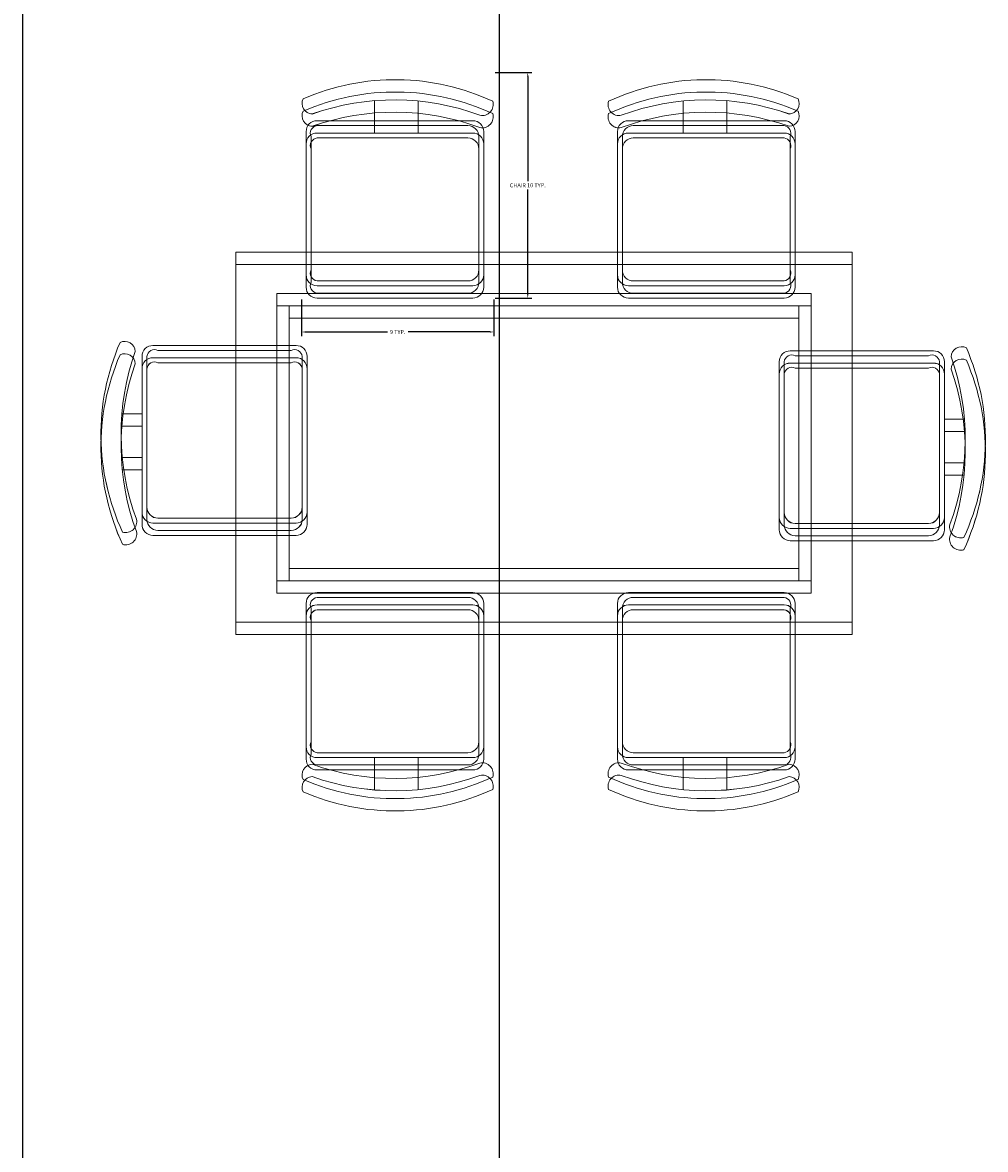
# Model space of a CAD drawing. Units: inches. Extents: x 2063 to 2617, y 1299 to 2210.
# Tile 18 of 22: x 2388 to 2431, y 1889 to 1939. Entities that reach past the tile are written whole.
import ezdxf

# ---------------------------------------------------------------- set-up
doc = ezdxf.new("R2010")
doc.units = ezdxf.units.IN
doc.layers.add('A-ANNO-DIMS', color=2, linetype='Continuous', lineweight=18)
doc.layers.add('A-FURN', color=8, linetype='Continuous', lineweight=18)
doc.styles.get("Standard").update_dxf_attribs({"font": 'arial.ttf'})
doc.dimstyles.get("Standard").update_dxf_attribs({"dimtxt": 0.18, "dimasz": 0.18, "dimexe": 0.18, "dimexo": 0.0625, "dimgap": 0.09, "dimtad": 0, "dimtih": 1, "dimtoh": 1, "dimdec": 4, "dimzin": 0, "dimdsep": 46, "dimtxsty": 'Standard', "dimcen": 0.09, "dimadec": 0, "dimazin": 0, "dimtfac": 1, "dimtdec": 4, "dimtofl": 0, "dimtmove": 0, "dimatfit": 3, "dimfxl": 1, "dimtolj": 1, "dimtzin": 0, "dimarcsym": 0})

# ---------------------------------------------------------------- blocks, each defined once
blk = doc.blocks.new('TABLE-DINING')
for points in [[(0, 17.017), (27.446, 17.017), (27.446, 0.549), (0, 0.549)], [(0, 17.017), (27.446, 17.017), (27.446, 0.549), (0, 0.549)], [(0, 17.016), (27.446, 17.016), (27.446, 0.549), (0, 0.549)], [(0, 17.016), (27.446, 17.016), (27.446, 0.549), (0, 0.549)], [(0, 16.468), (27.446, 16.468), (27.446, 0), (0, 0)], [(0, 16.468), (27.446, 16.468), (27.446, 0), (0, 0)], [(0, 16.467), (27.446, 16.467), (27.446, 0), (0, 0)], [(0, 16.467), (27.446, 16.467), (27.446, 0), (0, 0)], [(1.83, 15.187), (25.616, 15.187), (25.616, 2.379), (1.83, 2.379)], [(1.83, 15.187), (25.616, 15.187), (25.616, 2.379), (1.83, 2.379)], [(1.83, 15.187), (25.616, 15.187), (25.616, 2.379), (1.83, 2.379)], [(1.83, 15.187), (25.616, 15.187), (25.616, 2.379), (1.83, 2.379)], [(1.83, 14.638), (25.616, 14.638), (25.616, 1.83), (1.83, 1.83)], [(1.83, 14.638), (25.616, 14.638), (25.616, 1.83), (1.83, 1.83)], [(1.83, 14.638), (25.616, 14.638), (25.616, 1.83), (1.83, 1.83)], [(1.83, 14.638), (25.616, 14.638), (25.616, 1.83), (1.83, 1.83)], [(2.379, 14.638), (25.067, 14.638), (25.067, 2.928), (2.379, 2.928)], [(2.379, 14.638), (25.067, 14.638), (25.067, 2.927), (2.379, 2.927)], [(2.379, 14.638), (25.067, 14.638), (25.067, 2.928), (2.379, 2.928)], [(2.379, 14.638), (25.067, 14.638), (25.067, 2.927), (2.379, 2.927)], [(2.379, 14.089), (25.067, 14.089), (25.067, 2.379), (2.379, 2.379)], [(2.379, 14.089), (25.067, 14.089), (25.067, 2.379), (2.379, 2.379)], [(2.379, 14.089), (25.067, 14.089), (25.067, 2.379), (2.379, 2.379)], [(2.379, 14.089), (25.067, 14.089), (25.067, 2.379), (2.379, 2.379)]]:
    blk.add_lwpolyline(points, close=True)
blk = doc.blocks.new('CHAIR-DINING')
for points in [[(0.449, 8.202, -0.175809), (7.924, 8.145, 0.578392), (8.491, 8.768, 0.214524), (0.052, 8.881, 0.552014), (0.449, 8.202, -0.065079)], [(0.449, 8.201, -0.175809), (7.924, 8.145, 0.578392), (8.491, 8.767, 0.214524), (0.053, 8.881, 0.552014), (0.449, 8.201, -0.065079)], [(0.449, 8.202, -0.175809), (7.924, 8.145, 0.578392), (8.491, 8.768, 0.214524), (0.052, 8.881, 0.552014), (0.449, 8.202, -0.065079)], [(0.449, 8.201, -0.175809), (7.924, 8.145, 0.578392), (8.491, 8.767, 0.214524), (0.053, 8.881, 0.552014), (0.449, 8.201, -0.065079)], [(0.449, 7.653, -0.175809), (7.924, 7.596, 0.578392), (8.491, 8.219, 0.214524), (0.052, 8.332, 0.552014), (0.449, 7.653, -0.065079)], [(0.449, 7.652, -0.175809), (7.924, 7.596, 0.578392), (8.491, 8.218, 0.214524), (0.053, 8.332, 0.552014), (0.449, 7.652, -0.065079)], [(0.449, 7.653, -0.175809), (7.924, 7.596, 0.578392), (8.491, 8.219, 0.214524), (0.052, 8.332, 0.552014), (0.449, 7.653, -0.065079)], [(0.449, 7.652, -0.175809), (7.924, 7.596, 0.578392), (8.491, 8.218, 0.214524), (0.053, 8.332, 0.552014), (0.449, 7.652, -0.065079)], [(5.17, 7.902), (5.17, 8.779, -0.064759)], [(5.17, 7.901), (5.17, 8.779, -0.064759)], [(5.17, 7.902), (5.17, 8.779, -0.064759)], [(5.17, 7.901), (5.17, 8.779, -0.064759)], [(5.17, 7.353), (5.17, 8.23, -0.064759)], [(5.17, 7.352), (5.17, 8.23, -0.064759)], [(5.17, 7.353), (5.17, 8.23, -0.064759)], [(5.17, 7.352), (5.17, 8.23, -0.064759)], [(7.607, 7.902), (0.667, 7.902, 0.414214), (0.182, 7.416), (0.182, 1.035, 0.414214), (0.667, 0.549), (7.607, 0.549, 0.414214), (8.093, 1.035), (8.093, 7.416, 0.414214), (7.607, 7.902)], [(7.607, 7.902), (0.667, 7.902, 0.414214), (0.182, 7.416), (0.182, 1.035, 0.414214), (0.667, 0.549), (7.607, 0.549, 0.414214), (8.093, 1.035), (8.093, 7.416, 0.414214), (7.607, 7.902)], [(7.607, 7.901), (0.667, 7.901, 0.414214), (0.182, 7.416), (0.182, 1.035, 0.414214), (0.667, 0.549), (7.607, 0.549, 0.414214), (8.093, 1.035), (8.093, 7.416, 0.414214), (7.607, 7.901)], [(7.607, 7.901), (0.667, 7.901, 0.414214), (0.182, 7.416), (0.182, 1.035, 0.414214), (0.667, 0.549), (7.607, 0.549, 0.414214), (8.093, 1.035), (8.093, 7.416, 0.414214), (7.607, 7.901)], [(7.607, 7.353), (0.667, 7.353, 0.414214), (0.182, 6.867), (0.182, 0.486, 0.414214), (0.667, 0), (7.607, 0, 0.414214), (8.093, 0.486), (8.093, 6.867, 0.414214), (7.607, 7.353)], [(7.607, 7.353), (0.667, 7.353, 0.414214), (0.182, 6.867), (0.182, 0.486, 0.414214), (0.667, 0), (7.607, 0, 0.414214), (8.093, 0.486), (8.093, 6.867, 0.414214), (7.607, 7.353)], [(7.607, 7.352), (0.667, 7.352, 0.414214), (0.182, 6.867), (0.182, 0.486, 0.414214), (0.667, 0), (7.607, 0, 0.414214), (8.093, 0.486), (8.093, 6.867, 0.414214), (7.607, 7.352)], [(7.607, 7.352), (0.667, 7.352, 0.414214), (0.182, 6.867), (0.182, 0.486, 0.414214), (0.667, 0), (7.607, 0, 0.414214), (8.093, 0.486), (8.093, 6.867, 0.414214), (7.607, 7.352)]]:
    blk.add_lwpolyline(points, format="xyb")
for points in [[(3.227, 8.795), (3.227, 7.902)], [(3.227, 8.795), (3.227, 7.901)], [(3.227, 8.795), (3.227, 7.902)], [(3.227, 8.795), (3.227, 7.901)], [(3.227, 8.246), (3.227, 7.353)], [(3.227, 8.246), (3.227, 7.352)], [(3.227, 8.246), (3.227, 7.353)], [(3.227, 8.246), (3.227, 7.352)]]:
    blk.add_lwpolyline(points)
for points in [[(0.67, 7.683), (7.388, 7.683, -0.414214), (7.874, 7.197), (7.874, 1.254, -0.414214), (7.388, 0.768), (0.67, 0.768, -0.512069), (0.4, 1.254), (0.4, 7.197, -0.512069)], [(0.67, 7.683), (7.388, 7.683, -0.414214), (7.874, 7.197), (7.874, 1.253, -0.414214), (7.388, 0.768), (0.67, 0.768, -0.512069), (0.4, 1.253), (0.4, 7.197, -0.512069)], [(0.67, 7.683), (7.388, 7.683, -0.414214), (7.874, 7.197), (7.874, 1.254, -0.414214), (7.388, 0.768), (0.67, 0.768, -0.512069), (0.4, 1.254), (0.4, 7.197, -0.512069)], [(0.67, 7.683), (7.388, 7.683, -0.414214), (7.874, 7.197), (7.874, 1.253, -0.414214), (7.388, 0.768), (0.67, 0.768, -0.512069), (0.4, 1.253), (0.4, 7.197, -0.512069)], [(0.67, 7.134), (7.388, 7.134, -0.414214), (7.874, 6.648), (7.874, 0.705, -0.414214), (7.388, 0.219), (0.67, 0.219, -0.512069), (0.4, 0.705), (0.4, 6.648, -0.512069)], [(0.67, 7.134), (7.388, 7.134, -0.414214), (7.874, 6.648), (7.874, 0.704, -0.414214), (7.388, 0.219), (0.67, 0.219, -0.512069), (0.4, 0.704), (0.4, 6.648, -0.512069)], [(0.67, 7.134), (7.388, 7.134, -0.414214), (7.874, 6.648), (7.874, 0.705, -0.414214), (7.388, 0.219), (0.67, 0.219, -0.512069), (0.4, 0.705), (0.4, 6.648, -0.512069)], [(0.67, 7.134), (7.388, 7.134, -0.414214), (7.874, 6.648), (7.874, 0.704, -0.414214), (7.388, 0.219), (0.67, 0.219, -0.512069), (0.4, 0.704), (0.4, 6.648, -0.512069)]]:
    blk.add_lwpolyline(points, format="xyb", close=True)
blk = doc.blocks.new('*D27')
at = {"layer": 'A-ANNO-DIMS', "color": 0, "lineweight": -2, "transparency": 16777216}
for p, q in [((2409.206, 1936.746), (2410.831, 1936.746)), ((2410.651, 1936.566), (2410.651, 1931.903)), ((2410.651, 1926.874), (2410.651, 1931.537)), ((2409.206, 1926.694), (2410.831, 1926.694))]:
    blk.add_line(p, q, dxfattribs=at)
at = {"layer": 'A-ANNO-DIMS', "color": 0, "transparency": 16777216}
for points in [[(2410.621, 1936.566), (2410.681, 1936.566), (2410.651, 1936.746)], [(2410.621, 1926.874), (2410.681, 1926.874), (2410.651, 1926.694)]]:
    blk.add_solid(points, dxfattribs=at)
at = {"layer": 'Defpoints', "color": 0, "transparency": 16777216}
for p in [(2409.143, 1936.746), (2410.651, 1936.746), (2409.143, 1926.694)]:
    blk.add_point(p, dxfattribs=at)
at = {"layer": 'A-ANNO-DIMS', "color": 0, "transparency": 16777216, "insert": (2410.651, 1931.72), "char_height": 0.18, "attachment_point": 5}
blk.add_mtext('\\A1;CHAIR 10 TYP.', dxfattribs=at)
blk = doc.blocks.new('*D28')
at = {"layer": 'A-ANNO-DIMS', "color": 0, "lineweight": -2, "transparency": 16777216}
for p, q in [((2400.578, 1926.632), (2400.578, 1925.006)), ((2409.143, 1926.632), (2409.143, 1925.006)), ((2400.758, 1925.186), (2404.402, 1925.186)), ((2408.963, 1925.186), (2405.319, 1925.186))]:
    blk.add_line(p, q, dxfattribs=at)
at = {"layer": 'A-ANNO-DIMS', "color": 0, "transparency": 16777216}
for points in [[(2400.758, 1925.216), (2400.758, 1925.156), (2400.578, 1925.186)], [(2408.963, 1925.216), (2408.963, 1925.156), (2409.143, 1925.186)]]:
    blk.add_solid(points, dxfattribs=at)
at = {"layer": 'Defpoints', "color": 0, "transparency": 16777216}
for p in [(2400.578, 1926.694), (2409.143, 1926.694), (2409.143, 1925.186)]:
    blk.add_point(p, dxfattribs=at)
at = {"layer": 'A-ANNO-DIMS', "color": 0, "transparency": 16777216, "insert": (2404.861, 1925.186), "char_height": 0.18, "attachment_point": 5}
blk.add_mtext('\\A1;9 TYP.', dxfattribs=at)
blk = doc.blocks.new('*D55')
at = {"layer": 'A-ANNO-DIMS', "color": 0, "lineweight": -2, "transparency": 16777216}
for p, q in [((2388.15, 1975.75), (2388.15, 1317.702)), ((2409.375, 1975.75), (2409.375, 1317.702)), ((2388.33, 1317.882), (2398.297, 1317.882)), ((2409.195, 1317.882), (2399.229, 1317.882))]:
    blk.add_line(p, q, dxfattribs=at)
at = {"layer": 'A-ANNO-DIMS', "color": 0, "transparency": 16777216}
for points in [[(2388.33, 1317.912), (2388.33, 1317.852), (2388.15, 1317.882)], [(2409.195, 1317.912), (2409.195, 1317.852), (2409.375, 1317.882)]]:
    blk.add_solid(points, dxfattribs=at)
at = {"layer": 'Defpoints', "color": 0, "transparency": 16777216}
for p in [(2388.15, 1975.812), (2409.375, 1975.812), (2409.375, 1317.882)]:
    blk.add_point(p, dxfattribs=at)
at = {"layer": 'A-ANNO-DIMS', "color": 0, "transparency": 16777216, "insert": (2398.763, 1317.882), "char_height": 0.18, "attachment_point": 5}
blk.add_mtext('\\A1;21.225', dxfattribs=at)

msp = doc.modelspace()

# ---------------------------------------------------------------- linework, layer by layer
at = {"layer": 'A-FURN'}
for points in [[(2414.8171, 1934.839, -0.5783921), (2414.2508, 1935.4617, -0.2145244), (2422.689, 1935.5749, -0.552014), (2422.2925, 1934.8956, 0.1758092), (2414.8171, 1934.839)], [(2414.8171, 1934.839, -0.5783921), (2414.2508, 1935.4617, -0.2145244), (2422.689, 1935.5749, -0.552014), (2422.2925, 1934.8956, 0.1758092), (2414.8171, 1934.839)], [(2414.8171, 1934.8387, -0.5783921), (2414.2508, 1935.4614, -0.2145244), (2422.689, 1935.5746, -0.552014), (2422.2925, 1934.8953, 0.1758092), (2414.8171, 1934.8387)], [(2414.8171, 1934.8387, -0.5783921), (2414.2508, 1935.4614, -0.2145244), (2422.689, 1935.5746, -0.552014), (2422.2925, 1934.8953, 0.1758092), (2414.8171, 1934.8387)], [(2414.8171, 1934.2901, -0.5783921), (2414.2508, 1934.9128, -0.2145244), (2422.689, 1935.026, -0.552014), (2422.2925, 1934.3467, 0.1758092), (2414.8171, 1934.2901)], [(2414.8171, 1934.2901, -0.5783921), (2414.2508, 1934.9128, -0.2145244), (2422.689, 1935.026, -0.552014), (2422.2925, 1934.3467, 0.1758092), (2414.8171, 1934.2901)], [(2414.8171, 1934.2898, -0.5783921), (2414.2508, 1934.9125, -0.2145244), (2422.689, 1935.0257, -0.552014), (2422.2925, 1934.3464, 0.1758092), (2414.8171, 1934.2898)], [(2414.8171, 1934.2898, -0.5783921), (2414.2508, 1934.9125, -0.2145244), (2422.689, 1935.0257, -0.552014), (2422.2925, 1934.3464, 0.1758092), (2414.8171, 1934.2898)], [(2417.5719, 1934.5956), (2417.5719, 1935.4732, 0.0647586)], [(2417.5719, 1934.5956), (2417.5719, 1935.4732, 0.0647586)], [(2417.5719, 1934.5953), (2417.5719, 1935.473, 0.0647586)], [(2417.5719, 1934.5953), (2417.5719, 1935.473, 0.0647586)], [(2422.0742, 1934.5956, -0.4142136), (2422.5597, 1934.11), (2422.5597, 1927.7289, -0.4142136), (2422.0742, 1927.2434), (2415.1342, 1927.2434, -0.4142136), (2414.6487, 1927.7289), (2414.6487, 1934.11, -0.4142136), (2415.1342, 1934.5956), (2422.0742, 1934.5956)], [(2422.0742, 1934.5956, -0.4142136), (2422.5597, 1934.11), (2422.5597, 1927.7289, -0.4142136), (2422.0742, 1927.2434), (2415.1342, 1927.2434, -0.4142136), (2414.6487, 1927.7289), (2414.6487, 1934.11, -0.4142136), (2415.1342, 1934.5956), (2422.0742, 1934.5956)], [(2422.0742, 1934.5953, -0.4142136), (2422.5597, 1934.1097), (2422.5597, 1927.7286, -0.4142136), (2422.0742, 1927.2431), (2415.1343, 1927.2431, -0.4142136), (2414.6487, 1927.7286), (2414.6487, 1934.1097, -0.4142136), (2415.1343, 1934.5953), (2422.0742, 1934.5953)], [(2422.0742, 1934.5953, -0.4142136), (2422.5597, 1934.1097), (2422.5597, 1927.7286, -0.4142136), (2422.0742, 1927.2431), (2415.1343, 1927.2431, -0.4142136), (2414.6487, 1927.7286), (2414.6487, 1934.1097, -0.4142136), (2415.1343, 1934.5953), (2422.0742, 1934.5953)], [(2417.5719, 1934.0466), (2417.5719, 1934.9243, 0.0647586)], [(2417.5719, 1934.0466), (2417.5719, 1934.9243, 0.0647586)], [(2417.5719, 1934.0464), (2417.5719, 1934.924, 0.0647586)], [(2417.5719, 1934.0464), (2417.5719, 1934.924, 0.0647586)], [(2422.0742, 1934.0466, -0.4142136), (2422.5597, 1933.5611), (2422.5597, 1927.18, -0.4142136), (2422.0742, 1926.6944), (2415.1342, 1926.6944, -0.4142136), (2414.6487, 1927.18), (2414.6487, 1933.5611, -0.4142136), (2415.1342, 1934.0466), (2422.0742, 1934.0466)], [(2422.0742, 1934.0466, -0.4142136), (2422.5597, 1933.5611), (2422.5597, 1927.18, -0.4142136), (2422.0742, 1926.6944), (2415.1342, 1926.6944, -0.4142136), (2414.6487, 1927.18), (2414.6487, 1933.5611, -0.4142136), (2415.1342, 1934.0466), (2422.0742, 1934.0466)], [(2422.0742, 1934.0464, -0.4142136), (2422.5597, 1933.5608), (2422.5597, 1927.1797, -0.4142136), (2422.0742, 1926.6942), (2415.1343, 1926.6942, -0.4142136), (2414.6487, 1927.1797), (2414.6487, 1933.5608, -0.4142136), (2415.1343, 1934.0464), (2422.0742, 1934.0464)], [(2422.0742, 1934.0464, -0.4142136), (2422.5597, 1933.5608), (2422.5597, 1927.1797, -0.4142136), (2422.0742, 1926.6942), (2415.1343, 1926.6942, -0.4142136), (2414.6487, 1927.1797), (2414.6487, 1933.5608, -0.4142136), (2415.1343, 1934.0464), (2422.0742, 1934.0464)], [(2393.2276, 1916.8435, -0.5783921), (2392.6048, 1916.2772, -0.2145244), (2392.4916, 1924.7154, -0.552014), (2393.1709, 1924.319, 0.1758094), (2393.2276, 1916.8435)], [(2393.2276, 1916.8435, -0.5783921), (2392.6048, 1916.2772, -0.2145244), (2392.4916, 1924.7154, -0.552014), (2393.1709, 1924.319, 0.1758094), (2393.2276, 1916.8435)], [(2393.2276, 1916.8433, -0.5783921), (2392.6049, 1916.2769, -0.2145244), (2392.4916, 1924.7151, -0.552014), (2393.171, 1924.3187, 0.1758094), (2393.2276, 1916.8432)], [(2393.2276, 1916.8433, -0.5783921), (2392.6049, 1916.2769, -0.2145244), (2392.4916, 1924.7151, -0.552014), (2393.171, 1924.3187, 0.1758094), (2393.2276, 1916.8432)], [(2393.471, 1924.1006, -0.4142136), (2393.9565, 1924.5862), (2400.3376, 1924.5862, -0.4142136), (2400.8232, 1924.1006), (2400.8232, 1917.1607, -0.4142136), (2400.3376, 1916.6752), (2393.9565, 1916.6752, -0.4142136), (2393.471, 1917.1607), (2393.471, 1924.1006)], [(2393.471, 1924.1006, -0.4142136), (2393.9565, 1924.5862), (2400.3376, 1924.5862, -0.4142136), (2400.8232, 1924.1006), (2400.8232, 1917.1607, -0.4142136), (2400.3376, 1916.6752), (2393.9565, 1916.6752, -0.4142136), (2393.471, 1917.1607), (2393.471, 1924.1006)], [(2393.471, 1924.1003, -0.4142136), (2393.9565, 1924.5859), (2400.3377, 1924.5859, -0.4142136), (2400.8232, 1924.1003), (2400.8232, 1917.1604, -0.4142136), (2400.3377, 1916.6749), (2393.9565, 1916.6749, -0.4142136), (2393.471, 1917.1604), (2393.471, 1924.1003)], [(2393.471, 1924.1003, -0.4142136), (2393.9565, 1924.5859), (2400.3377, 1924.5859, -0.4142136), (2400.8232, 1924.1003), (2400.8232, 1917.1604, -0.4142136), (2400.3377, 1916.6749), (2393.9565, 1916.6749, -0.4142136), (2393.471, 1917.1604), (2393.471, 1924.1003)], [(2429.5085, 1924.0813, -0.1758092), (2429.4519, 1916.6059, 0.5783921), (2430.0746, 1916.0395, 0.2145244), (2430.1878, 1924.4777, 0.552014), (2429.5085, 1924.0813, -0.065079)], [(2429.5085, 1924.0813, -0.1758092), (2429.4519, 1916.6059, 0.5783921), (2430.0746, 1916.0395, 0.2145244), (2430.1878, 1924.4777, 0.552014), (2429.5085, 1924.0813, -0.065079)], [(2429.5085, 1924.081, -0.1758092), (2429.4519, 1916.6056, 0.5783921), (2430.0746, 1916.0392, 0.2145244), (2430.1878, 1924.4774, 0.552014), (2429.5085, 1924.081, -0.065079)], [(2429.5085, 1924.081, -0.1758092), (2429.4519, 1916.6056, 0.5783921), (2430.0746, 1916.0392, 0.2145244), (2430.1878, 1924.4774, 0.552014), (2429.5085, 1924.081, -0.065079)], [(2393.2276, 1916.2946, -0.5783921), (2392.6048, 1915.7283, -0.2145244), (2392.4916, 1924.1665, -0.552014), (2393.1709, 1923.7701, 0.1758094), (2393.2276, 1916.2946)], [(2393.2276, 1916.2946, -0.5783921), (2392.6048, 1915.7283, -0.2145244), (2392.4916, 1924.1665, -0.552014), (2393.1709, 1923.7701, 0.1758094), (2393.2276, 1916.2946)], [(2393.2276, 1916.2943, -0.5783921), (2392.6049, 1915.728, -0.2145244), (2392.4916, 1924.1662, -0.552014), (2393.171, 1923.7698, 0.1758094), (2393.2276, 1916.2943)], [(2393.2276, 1916.2943, -0.5783921), (2392.6049, 1915.728, -0.2145244), (2392.4916, 1924.1662, -0.552014), (2393.171, 1923.7698, 0.1758094), (2393.2276, 1916.2943)], [(2393.471, 1923.5517, -0.4142136), (2393.9565, 1924.0372), (2400.3376, 1924.0372, -0.4142136), (2400.8232, 1923.5517), (2400.8232, 1916.6118, -0.4142136), (2400.3376, 1916.1262), (2393.9565, 1916.1262, -0.4142136), (2393.471, 1916.6118), (2393.471, 1923.5517)], [(2393.471, 1923.5517, -0.4142136), (2393.9565, 1924.0372), (2400.3376, 1924.0372, -0.4142136), (2400.8232, 1923.5517), (2400.8232, 1916.6118, -0.4142136), (2400.3376, 1916.1262), (2393.9565, 1916.1262, -0.4142136), (2393.471, 1916.6118), (2393.471, 1923.5517)], [(2393.471, 1923.5514, -0.4142136), (2393.9565, 1924.037), (2400.3377, 1924.037, -0.4142136), (2400.8232, 1923.5514), (2400.8232, 1916.6115, -0.4142136), (2400.3377, 1916.126), (2393.9565, 1916.126, -0.4142136), (2393.471, 1916.6115), (2393.471, 1923.5514)], [(2393.471, 1923.5514, -0.4142136), (2393.9565, 1924.037), (2400.3377, 1924.037, -0.4142136), (2400.8232, 1923.5514), (2400.8232, 1916.6115, -0.4142136), (2400.3377, 1916.126), (2393.9565, 1916.126, -0.4142136), (2393.471, 1916.6115), (2393.471, 1923.5514)], [(2429.2084, 1923.863, 0.4142136), (2428.7229, 1924.3485), (2422.3418, 1924.3485, 0.4142136), (2421.8562, 1923.863), (2421.8562, 1916.923, 0.4142136), (2422.3418, 1916.4375), (2428.7229, 1916.4375, 0.4142136), (2429.2084, 1916.923), (2429.2084, 1923.863)], [(2429.2084, 1923.863, 0.4142136), (2428.7229, 1924.3485), (2422.3418, 1924.3485, 0.4142136), (2421.8562, 1923.863), (2421.8562, 1916.923, 0.4142136), (2422.3418, 1916.4375), (2428.7229, 1916.4375, 0.4142136), (2429.2084, 1916.923), (2429.2084, 1923.863)], [(2429.2085, 1923.8627, 0.4142136), (2428.7229, 1924.3482), (2422.3418, 1924.3482, 0.4142136), (2421.8563, 1923.8627), (2421.8563, 1916.9227, 0.4142136), (2422.3418, 1916.4372), (2428.7229, 1916.4372, 0.4142136), (2429.2085, 1916.9227), (2429.2085, 1923.8627)], [(2429.2085, 1923.8627, 0.4142136), (2428.7229, 1924.3482), (2422.3418, 1924.3482, 0.4142136), (2421.8563, 1923.8627), (2421.8563, 1916.9227, 0.4142136), (2422.3418, 1916.4372), (2428.7229, 1916.4372, 0.4142136), (2429.2085, 1916.9227), (2429.2085, 1923.8627)], [(2429.5085, 1923.5324, -0.1758092), (2429.4519, 1916.0569, 0.5783921), (2430.0746, 1915.4906, 0.2145244), (2430.1878, 1923.9288, 0.552014), (2429.5085, 1923.5324, -0.065079)], [(2429.5085, 1923.5324, -0.1758092), (2429.4519, 1916.0569, 0.5783921), (2430.0746, 1915.4906, 0.2145244), (2430.1878, 1923.9288, 0.552014), (2429.5085, 1923.5324, -0.065079)], [(2429.5085, 1923.5321, -0.1758092), (2429.4519, 1916.0567, 0.5783921), (2430.0746, 1915.4903, 0.2145244), (2430.1878, 1923.9285, 0.552014), (2429.5085, 1923.5321, -0.065079)], [(2429.5085, 1923.5321, -0.1758092), (2429.4519, 1916.0567, 0.5783921), (2430.0746, 1915.4903, 0.2145244), (2430.1878, 1923.9285, 0.552014), (2429.5085, 1923.5321, -0.065079)], [(2429.2084, 1923.314, 0.4142136), (2428.7229, 1923.7996), (2422.3418, 1923.7996, 0.4142136), (2421.8562, 1923.314), (2421.8562, 1916.3741, 0.4142136), (2422.3418, 1915.8886), (2428.7229, 1915.8886, 0.4142136), (2429.2084, 1916.3741), (2429.2084, 1923.314)], [(2429.2084, 1923.314, 0.4142136), (2428.7229, 1923.7996), (2422.3418, 1923.7996, 0.4142136), (2421.8562, 1923.314), (2421.8562, 1916.3741, 0.4142136), (2422.3418, 1915.8886), (2428.7229, 1915.8886, 0.4142136), (2429.2084, 1916.3741), (2429.2084, 1923.314)], [(2429.2085, 1923.3138, 0.4142136), (2428.7229, 1923.7993), (2422.3418, 1923.7993, 0.4142136), (2421.8563, 1923.3138), (2421.8563, 1916.3738, 0.4142136), (2422.3418, 1915.8883), (2428.7229, 1915.8883, 0.4142136), (2429.2085, 1916.3738), (2429.2085, 1923.3138)], [(2429.2085, 1923.3138, 0.4142136), (2428.7229, 1923.7993), (2422.3418, 1923.7993, 0.4142136), (2421.8563, 1923.3138), (2421.8563, 1916.3738, 0.4142136), (2422.3418, 1915.8883), (2428.7229, 1915.8883, 0.4142136), (2429.2085, 1916.3738), (2429.2085, 1923.3138)], [(2393.471, 1919.5983), (2392.5933, 1919.5983, 0.0647586)], [(2393.471, 1919.5983), (2392.5933, 1919.5983, 0.0647586)], [(2393.471, 1919.5981), (2392.5933, 1919.5981, 0.0647586)], [(2393.471, 1919.5981), (2392.5933, 1919.5981, 0.0647586)], [(2393.471, 1919.0494), (2392.5933, 1919.0494, 0.0647586)], [(2393.471, 1919.0494), (2392.5933, 1919.0494, 0.0647586)], [(2393.471, 1919.0491), (2392.5933, 1919.0491, 0.0647586)], [(2393.471, 1919.0491), (2392.5933, 1919.0491, 0.0647586)], [(2429.2084, 1919.3607), (2430.0861, 1919.3607, -0.0647586)], [(2429.2084, 1919.3607), (2430.0861, 1919.3607, -0.0647586)], [(2429.2085, 1919.3604), (2430.0861, 1919.3604, -0.0647586)], [(2429.2085, 1919.3604), (2430.0861, 1919.3604, -0.0647586)], [(2429.2084, 1918.8118), (2430.0861, 1918.8118, -0.0647586)], [(2429.2084, 1918.8118), (2430.0861, 1918.8118, -0.0647586)], [(2429.2085, 1918.8115), (2430.0861, 1918.8115, -0.0647586)], [(2429.2085, 1918.8115), (2430.0861, 1918.8115, -0.0647586)], [(2408.2066, 1906.2298), (2401.2666, 1906.2298, -0.4142136), (2400.7811, 1906.7153), (2400.7811, 1913.0965, -0.4142136), (2401.2666, 1913.582), (2408.2066, 1913.582, -0.4142136), (2408.6921, 1913.0965), (2408.6921, 1906.7153, -0.4142136), (2408.2066, 1906.2298)], [(2408.2066, 1906.2298), (2401.2666, 1906.2298, -0.4142136), (2400.7811, 1906.7153), (2400.7811, 1913.0965, -0.4142136), (2401.2666, 1913.582), (2408.2066, 1913.582, -0.4142136), (2408.6921, 1913.0965), (2408.6921, 1906.7153, -0.4142136), (2408.2066, 1906.2298)], [(2408.2066, 1906.2295), (2401.2667, 1906.2295, -0.4142136), (2400.7811, 1906.715), (2400.7811, 1913.0962, -0.4142136), (2401.2667, 1913.5817), (2408.2066, 1913.5817, -0.4142136), (2408.6921, 1913.0962), (2408.6921, 1906.715, -0.4142136), (2408.2066, 1906.2295)], [(2408.2066, 1906.2295), (2401.2667, 1906.2295, -0.4142136), (2400.7811, 1906.715), (2400.7811, 1913.0962, -0.4142136), (2401.2667, 1913.5817), (2408.2066, 1913.5817, -0.4142136), (2408.6921, 1913.0962), (2408.6921, 1906.715, -0.4142136), (2408.2066, 1906.2295)], [(2422.0742, 1906.2298, 0.4142136), (2422.5597, 1906.7153), (2422.5597, 1913.0965, 0.4142136), (2422.0742, 1913.582), (2415.1342, 1913.582, 0.4142136), (2414.6487, 1913.0965), (2414.6487, 1906.7153, 0.4142136), (2415.1342, 1906.2298), (2422.0742, 1906.2298)], [(2422.0742, 1906.2298, 0.4142136), (2422.5597, 1906.7153), (2422.5597, 1913.0965, 0.4142136), (2422.0742, 1913.582), (2415.1342, 1913.582, 0.4142136), (2414.6487, 1913.0965), (2414.6487, 1906.7153, 0.4142136), (2415.1342, 1906.2298), (2422.0742, 1906.2298)], [(2422.0742, 1906.2295, 0.4142136), (2422.5597, 1906.715), (2422.5597, 1913.0962, 0.4142136), (2422.0742, 1913.5817), (2415.1343, 1913.5817, 0.4142136), (2414.6487, 1913.0962), (2414.6487, 1906.715, 0.4142136), (2415.1343, 1906.2295), (2422.0742, 1906.2295)], [(2422.0742, 1906.2295, 0.4142136), (2422.5597, 1906.715), (2422.5597, 1913.0962, 0.4142136), (2422.0742, 1913.5817), (2415.1343, 1913.5817, 0.4142136), (2414.6487, 1913.0962), (2414.6487, 1906.715, 0.4142136), (2415.1343, 1906.2295), (2422.0742, 1906.2295)], [(2408.2066, 1905.6809), (2401.2666, 1905.6809, -0.4142136), (2400.7811, 1906.1664), (2400.7811, 1912.5476, -0.4142136), (2401.2666, 1913.0331), (2408.2066, 1913.0331, -0.4142136), (2408.6921, 1912.5476), (2408.6921, 1906.1664, -0.4142136), (2408.2066, 1905.6809)], [(2408.2066, 1905.6809), (2401.2666, 1905.6809, -0.4142136), (2400.7811, 1906.1664), (2400.7811, 1912.5476, -0.4142136), (2401.2666, 1913.0331), (2408.2066, 1913.0331, -0.4142136), (2408.6921, 1912.5476), (2408.6921, 1906.1664, -0.4142136), (2408.2066, 1905.6809)], [(2408.2066, 1905.6806), (2401.2667, 1905.6806, -0.4142136), (2400.7811, 1906.1661), (2400.7811, 1912.5473, -0.4142136), (2401.2667, 1913.0328), (2408.2066, 1913.0328, -0.4142136), (2408.6921, 1912.5473), (2408.6921, 1906.1661, -0.4142136), (2408.2066, 1905.6806)], [(2408.2066, 1905.6806), (2401.2667, 1905.6806, -0.4142136), (2400.7811, 1906.1661), (2400.7811, 1912.5473, -0.4142136), (2401.2667, 1913.0328), (2408.2066, 1913.0328, -0.4142136), (2408.6921, 1912.5473), (2408.6921, 1906.1661, -0.4142136), (2408.2066, 1905.6806)], [(2422.0742, 1905.6809, 0.4142136), (2422.5597, 1906.1664), (2422.5597, 1912.5476, 0.4142136), (2422.0742, 1913.0331), (2415.1342, 1913.0331, 0.4142136), (2414.6487, 1912.5476), (2414.6487, 1906.1664, 0.4142136), (2415.1342, 1905.6809), (2422.0742, 1905.6809)], [(2422.0742, 1905.6809, 0.4142136), (2422.5597, 1906.1664), (2422.5597, 1912.5476, 0.4142136), (2422.0742, 1913.0331), (2415.1342, 1913.0331, 0.4142136), (2414.6487, 1912.5476), (2414.6487, 1906.1664, 0.4142136), (2415.1342, 1905.6809), (2422.0742, 1905.6809)], [(2422.0742, 1905.6806, 0.4142136), (2422.5597, 1906.1661), (2422.5597, 1912.5473, 0.4142136), (2422.0742, 1913.0328), (2415.1343, 1913.0328, 0.4142136), (2414.6487, 1912.5473), (2414.6487, 1906.1661, 0.4142136), (2415.1343, 1905.6806), (2422.0742, 1905.6806)], [(2422.0742, 1905.6806, 0.4142136), (2422.5597, 1906.1661), (2422.5597, 1912.5473, 0.4142136), (2422.0742, 1913.0328), (2415.1343, 1913.0328, 0.4142136), (2414.6487, 1912.5473), (2414.6487, 1906.1661, 0.4142136), (2415.1343, 1905.6806), (2422.0742, 1905.6806)], [(2408.5237, 1905.9864, -0.5783921), (2409.0901, 1905.3637, -0.2145244), (2400.6519, 1905.2505, -0.552014), (2401.0483, 1905.9298, 0.1758093), (2408.5237, 1905.9864)], [(2408.5237, 1905.9864, -0.5783921), (2409.0901, 1905.3637, -0.2145244), (2400.6519, 1905.2505, -0.552014), (2401.0483, 1905.9298, 0.1758093), (2408.5237, 1905.9864)], [(2408.5237, 1905.9861, -0.5783921), (2409.0901, 1905.3634, -0.2145244), (2400.6519, 1905.2502, -0.552014), (2401.0483, 1905.9295, 0.1758093), (2408.5237, 1905.9861)], [(2408.5237, 1905.9861, -0.5783921), (2409.0901, 1905.3634, -0.2145244), (2400.6519, 1905.2502, -0.552014), (2401.0483, 1905.9295, 0.1758093), (2408.5237, 1905.9861)], [(2405.7689, 1906.2298), (2405.7689, 1905.3521, 0.0647586)], [(2405.7689, 1906.2298), (2405.7689, 1905.3521, 0.0647586)], [(2405.7689, 1906.2295), (2405.7689, 1905.3518, 0.0647586)], [(2405.7689, 1906.2295), (2405.7689, 1905.3518, 0.0647586)], [(2422.2925, 1905.9298, -0.1758093), (2414.8171, 1905.9864, 0.5783921), (2414.2508, 1905.3637, 0.2145244), (2422.689, 1905.2505, 0.552014), (2422.2925, 1905.9298, -0.065079)], [(2422.2925, 1905.9298, -0.1758093), (2414.8171, 1905.9864, 0.5783921), (2414.2508, 1905.3637, 0.2145244), (2422.689, 1905.2505, 0.552014), (2422.2925, 1905.9298, -0.065079)], [(2422.2925, 1905.9295, -0.1758093), (2414.8171, 1905.9861, 0.5783921), (2414.2508, 1905.3634, 0.2145244), (2422.689, 1905.2502, 0.552014), (2422.2925, 1905.9295, -0.065079)], [(2422.2925, 1905.9295, -0.1758093), (2414.8171, 1905.9861, 0.5783921), (2414.2508, 1905.3634, 0.2145244), (2422.689, 1905.2502, 0.552014), (2422.2925, 1905.9295, -0.065079)], [(2417.5719, 1906.2298), (2417.5719, 1905.3521, -0.0647586)], [(2417.5719, 1906.2298), (2417.5719, 1905.3521, -0.0647586)], [(2417.5719, 1906.2295), (2417.5719, 1905.3518, -0.0647586)], [(2417.5719, 1906.2295), (2417.5719, 1905.3518, -0.0647586)], [(2408.5237, 1905.4375, -0.5783921), (2409.0901, 1904.8148, -0.2145244), (2400.6519, 1904.7015, -0.552014), (2401.0483, 1905.3809, 0.1758093), (2408.5237, 1905.4375)], [(2408.5237, 1905.4375, -0.5783921), (2409.0901, 1904.8148, -0.2145244), (2400.6519, 1904.7015, -0.552014), (2401.0483, 1905.3809, 0.1758093), (2408.5237, 1905.4375)], [(2408.5237, 1905.4372, -0.5783921), (2409.0901, 1904.8145, -0.2145244), (2400.6519, 1904.7012, -0.552014), (2401.0483, 1905.3806, 0.1758093), (2408.5237, 1905.4372)], [(2408.5237, 1905.4372, -0.5783921), (2409.0901, 1904.8145, -0.2145244), (2400.6519, 1904.7012, -0.552014), (2401.0483, 1905.3806, 0.1758093), (2408.5237, 1905.4372)], [(2405.7689, 1905.6809), (2405.7689, 1904.8032, 0.0647586)], [(2405.7689, 1905.6809), (2405.7689, 1904.8032, 0.0647586)], [(2405.7689, 1905.6806), (2405.7689, 1904.8029, 0.0647586)], [(2405.7689, 1905.6806), (2405.7689, 1904.8029, 0.0647586)], [(2422.2925, 1905.3809, -0.1758093), (2414.8171, 1905.4375, 0.5783921), (2414.2508, 1904.8148, 0.2145244), (2422.689, 1904.7015, 0.552014), (2422.2925, 1905.3809, -0.065079)], [(2422.2925, 1905.3809, -0.1758093), (2414.8171, 1905.4375, 0.5783921), (2414.2508, 1904.8148, 0.2145244), (2422.689, 1904.7015, 0.552014), (2422.2925, 1905.3809, -0.065079)], [(2422.2925, 1905.3806, -0.1758093), (2414.8171, 1905.4372, 0.5783921), (2414.2508, 1904.8145, 0.2145244), (2422.689, 1904.7012, 0.552014), (2422.2925, 1905.3806, -0.065079)], [(2422.2925, 1905.3806, -0.1758093), (2414.8171, 1905.4372, 0.5783921), (2414.2508, 1904.8145, 0.2145244), (2422.689, 1904.7012, 0.552014), (2422.2925, 1905.3806, -0.065079)], [(2417.5719, 1905.6809), (2417.5719, 1904.8032, -0.0647586)], [(2417.5719, 1905.6809), (2417.5719, 1904.8032, -0.0647586)], [(2417.5719, 1905.6806), (2417.5719, 1904.8029, -0.0647586)], [(2417.5719, 1905.6806), (2417.5719, 1904.8029, -0.0647586)]]:
    msp.add_lwpolyline(points, format="xyb", dxfattribs=at)
for points in [[(2419.5145, 1935.4892), (2419.5145, 1934.5956)], [(2419.5145, 1935.4892), (2419.5145, 1934.5956)], [(2419.5145, 1935.4889), (2419.5145, 1934.5953)], [(2419.5145, 1935.4889), (2419.5145, 1934.5953)], [(2419.5145, 1934.9403), (2419.5145, 1934.0466)], [(2419.5145, 1934.9403), (2419.5145, 1934.0466)], [(2419.5145, 1934.94), (2419.5145, 1934.0464)], [(2419.5145, 1934.94), (2419.5145, 1934.0464)], [(2392.5773, 1921.5409), (2393.471, 1921.5409)], [(2392.5773, 1921.5409), (2393.471, 1921.5409)], [(2392.5774, 1921.5407), (2393.471, 1921.5407)], [(2392.5774, 1921.5407), (2393.471, 1921.5407)], [(2392.5773, 1920.992), (2393.471, 1920.992)], [(2392.5773, 1920.992), (2393.471, 1920.992)], [(2392.5774, 1920.9917), (2393.471, 1920.9917)], [(2392.5774, 1920.9917), (2393.471, 1920.9917)], [(2430.1021, 1921.3033), (2429.2084, 1921.3033)], [(2430.1021, 1921.3033), (2429.2084, 1921.3033)], [(2430.1021, 1921.303), (2429.2085, 1921.303)], [(2430.1021, 1921.303), (2429.2085, 1921.303)], [(2430.1021, 1920.7543), (2429.2084, 1920.7543)], [(2430.1021, 1920.7543), (2429.2084, 1920.7543)], [(2430.1021, 1920.7541), (2429.2085, 1920.7541)], [(2430.1021, 1920.7541), (2429.2085, 1920.7541)], [(2403.8263, 1905.3362), (2403.8263, 1906.2298)], [(2403.8263, 1905.3362), (2403.8263, 1906.2298)], [(2403.8263, 1905.3359), (2403.8263, 1906.2295)], [(2403.8263, 1905.3359), (2403.8263, 1906.2295)], [(2419.5145, 1905.3362), (2419.5145, 1906.2298)], [(2419.5145, 1905.3362), (2419.5145, 1906.2298)], [(2419.5145, 1905.3359), (2419.5145, 1906.2295)], [(2419.5145, 1905.3359), (2419.5145, 1906.2295)], [(2403.8263, 1904.7873), (2403.8263, 1905.6809)], [(2403.8263, 1904.7873), (2403.8263, 1905.6809)], [(2403.8263, 1904.787), (2403.8263, 1905.6806)], [(2403.8263, 1904.787), (2403.8263, 1905.6806)], [(2419.5145, 1904.7873), (2419.5145, 1905.6809)], [(2419.5145, 1904.7873), (2419.5145, 1905.6809)], [(2419.5145, 1904.787), (2419.5145, 1905.6806)], [(2419.5145, 1904.787), (2419.5145, 1905.6806)]]:
    msp.add_lwpolyline(points, dxfattribs=at)
for points in [[(2422.0712, 1934.3768), (2415.353, 1934.3768, 0.4142136), (2414.8674, 1933.8913), (2414.8674, 1927.9476, 0.4142136), (2415.353, 1927.4621), (2422.0712, 1927.4621, 0.5120695), (2422.341, 1927.9476), (2422.341, 1933.8913, 0.5120695)], [(2422.0712, 1934.3768), (2415.353, 1934.3768, 0.4142136), (2414.8674, 1933.8913), (2414.8674, 1927.9476, 0.4142136), (2415.353, 1927.4621), (2422.0712, 1927.4621, 0.5120695), (2422.341, 1927.9476), (2422.341, 1933.8913, 0.5120695)], [(2422.0713, 1934.3765), (2415.353, 1934.3765, 0.4142136), (2414.8675, 1933.891), (2414.8675, 1927.9473, 0.4142136), (2415.353, 1927.4618), (2422.0713, 1927.4618, 0.5120695), (2422.341, 1927.9473), (2422.341, 1933.891, 0.5120695)], [(2422.0713, 1934.3765), (2415.353, 1934.3765, 0.4142136), (2414.8675, 1933.891), (2414.8675, 1927.9473, 0.4142136), (2415.353, 1927.4618), (2422.0713, 1927.4618, 0.5120695), (2422.341, 1927.9473), (2422.341, 1933.891, 0.5120695)], [(2422.0712, 1933.8279), (2415.353, 1933.8279, 0.4142136), (2414.8674, 1933.3424), (2414.8674, 1927.3987, 0.4142136), (2415.353, 1926.9132), (2422.0712, 1926.9132, 0.5120695), (2422.341, 1927.3987), (2422.341, 1933.3424, 0.5120695)], [(2422.0712, 1933.8279), (2415.353, 1933.8279, 0.4142136), (2414.8674, 1933.3424), (2414.8674, 1927.3987, 0.4142136), (2415.353, 1926.9132), (2422.0712, 1926.9132, 0.5120695), (2422.341, 1927.3987), (2422.341, 1933.3424, 0.5120695)], [(2422.0713, 1933.8276), (2415.353, 1933.8276, 0.4142136), (2414.8675, 1933.3421), (2414.8675, 1927.3984, 0.4142136), (2415.353, 1926.9129), (2422.0713, 1926.9129, 0.5120695), (2422.341, 1927.3984), (2422.341, 1933.3421, 0.5120695)], [(2422.0713, 1933.8276), (2415.353, 1933.8276, 0.4142136), (2414.8675, 1933.3421), (2414.8675, 1927.3984, 0.4142136), (2415.353, 1926.9129), (2422.0713, 1926.9129, 0.5120695), (2422.341, 1927.3984), (2422.341, 1933.3421, 0.5120695)], [(2393.6897, 1924.0977), (2393.6897, 1917.3794, 0.4142136), (2394.1752, 1916.8939), (2400.1189, 1916.8939, 0.4142136), (2400.6044, 1917.3794), (2400.6044, 1924.0977, 0.5120695), (2400.1189, 1924.3674), (2394.1752, 1924.3674, 0.5120695)], [(2393.6897, 1924.0977), (2393.6897, 1917.3794, 0.4142136), (2394.1752, 1916.8939), (2400.1189, 1916.8939, 0.4142136), (2400.6044, 1917.3794), (2400.6044, 1924.0977, 0.5120695), (2400.1189, 1924.3674), (2394.1752, 1924.3674, 0.5120695)], [(2393.6897, 1924.0974), (2393.6897, 1917.3791, 0.4142136), (2394.1752, 1916.8936), (2400.1189, 1916.8936, 0.4142136), (2400.6045, 1917.3791), (2400.6045, 1924.0974, 0.5120695), (2400.1189, 1924.3671), (2394.1752, 1924.3671, 0.5120695)], [(2393.6897, 1924.0974), (2393.6897, 1917.3791, 0.4142136), (2394.1752, 1916.8936), (2400.1189, 1916.8936, 0.4142136), (2400.6045, 1917.3791), (2400.6045, 1924.0974, 0.5120695), (2400.1189, 1924.3671), (2394.1752, 1924.3671, 0.5120695)], [(2428.9897, 1923.86), (2428.9897, 1917.1417, -0.4142136), (2428.5042, 1916.6562), (2422.5605, 1916.6562, -0.4142136), (2422.075, 1917.1417), (2422.075, 1923.86, -0.5120695), (2422.5605, 1924.1297), (2428.5042, 1924.1297, -0.5120695)], [(2428.9897, 1923.86), (2428.9897, 1917.1417, -0.4142136), (2428.5042, 1916.6562), (2422.5605, 1916.6562, -0.4142136), (2422.075, 1917.1417), (2422.075, 1923.86, -0.5120695), (2422.5605, 1924.1297), (2428.5042, 1924.1297, -0.5120695)], [(2428.9897, 1923.8597), (2428.9897, 1917.1415, -0.4142136), (2428.5042, 1916.6559), (2422.5605, 1916.6559, -0.4142136), (2422.075, 1917.1415), (2422.075, 1923.8597, -0.5120695), (2422.5605, 1924.1295), (2428.5042, 1924.1295, -0.5120695)], [(2428.9897, 1923.8597), (2428.9897, 1917.1415, -0.4142136), (2428.5042, 1916.6559), (2422.5605, 1916.6559, -0.4142136), (2422.075, 1917.1415), (2422.075, 1923.8597, -0.5120695), (2422.5605, 1924.1295), (2428.5042, 1924.1295, -0.5120695)], [(2393.6897, 1923.5488), (2393.6897, 1916.8305, 0.4142136), (2394.1752, 1916.345), (2400.1189, 1916.345, 0.4142136), (2400.6044, 1916.8305), (2400.6044, 1923.5488, 0.5120695), (2400.1189, 1923.8185), (2394.1752, 1923.8185, 0.5120695)], [(2393.6897, 1923.5488), (2393.6897, 1916.8305, 0.4142136), (2394.1752, 1916.345), (2400.1189, 1916.345, 0.4142136), (2400.6044, 1916.8305), (2400.6044, 1923.5488, 0.5120695), (2400.1189, 1923.8185), (2394.1752, 1923.8185, 0.5120695)], [(2393.6897, 1923.5485), (2393.6897, 1916.8302, 0.4142136), (2394.1752, 1916.3447), (2400.1189, 1916.3447, 0.4142136), (2400.6045, 1916.8302), (2400.6045, 1923.5485, 0.5120695), (2400.1189, 1923.8182), (2394.1752, 1923.8182, 0.5120695)], [(2393.6897, 1923.5485), (2393.6897, 1916.8302, 0.4142136), (2394.1752, 1916.3447), (2400.1189, 1916.3447, 0.4142136), (2400.6045, 1916.8302), (2400.6045, 1923.5485, 0.5120695), (2400.1189, 1923.8182), (2394.1752, 1923.8182, 0.5120695)], [(2428.9897, 1923.3111), (2428.9897, 1916.5928, -0.4142136), (2428.5042, 1916.1073), (2422.5605, 1916.1073, -0.4142136), (2422.075, 1916.5928), (2422.075, 1923.3111, -0.5120695), (2422.5605, 1923.5808), (2428.5042, 1923.5808, -0.5120695)], [(2428.9897, 1923.3111), (2428.9897, 1916.5928, -0.4142136), (2428.5042, 1916.1073), (2422.5605, 1916.1073, -0.4142136), (2422.075, 1916.5928), (2422.075, 1923.3111, -0.5120695), (2422.5605, 1923.5808), (2428.5042, 1923.5808, -0.5120695)], [(2428.9897, 1923.3108), (2428.9897, 1916.5925, -0.4142136), (2428.5042, 1916.107), (2422.5605, 1916.107, -0.4142136), (2422.075, 1916.5925), (2422.075, 1923.3108, -0.5120695), (2422.5605, 1923.5805), (2428.5042, 1923.5805, -0.5120695)], [(2428.9897, 1923.3108), (2428.9897, 1916.5925, -0.4142136), (2428.5042, 1916.107), (2422.5605, 1916.107, -0.4142136), (2422.075, 1916.5925), (2422.075, 1923.3108, -0.5120695), (2422.5605, 1923.5805), (2428.5042, 1923.5805, -0.5120695)], [(2401.2696, 1906.4485), (2407.9879, 1906.4485, 0.4142136), (2408.4734, 1906.9341), (2408.4734, 1912.8777, 0.4142136), (2407.9879, 1913.3633), (2401.2696, 1913.3633, 0.5120695), (2400.9998, 1912.8777), (2400.9998, 1906.9341, 0.5120695)], [(2401.2696, 1906.4485), (2407.9879, 1906.4485, 0.4142136), (2408.4734, 1906.9341), (2408.4734, 1912.8777, 0.4142136), (2407.9879, 1913.3633), (2401.2696, 1913.3633, 0.5120695), (2400.9998, 1912.8777), (2400.9998, 1906.9341, 0.5120695)], [(2401.2696, 1906.4483), (2407.9879, 1906.4483, 0.4142136), (2408.4734, 1906.9338), (2408.4734, 1912.8775, 0.4142136), (2407.9879, 1913.363), (2401.2696, 1913.363, 0.5120695), (2400.9999, 1912.8775), (2400.9999, 1906.9338, 0.5120695)], [(2401.2696, 1906.4483), (2407.9879, 1906.4483, 0.4142136), (2408.4734, 1906.9338), (2408.4734, 1912.8775, 0.4142136), (2407.9879, 1913.363), (2401.2696, 1913.363, 0.5120695), (2400.9999, 1912.8775), (2400.9999, 1906.9338, 0.5120695)], [(2422.0712, 1906.4485), (2415.353, 1906.4485, -0.4142136), (2414.8674, 1906.9341), (2414.8674, 1912.8777, -0.4142136), (2415.353, 1913.3633), (2422.0712, 1913.3633, -0.5120695), (2422.341, 1912.8777), (2422.341, 1906.9341, -0.5120695)], [(2422.0712, 1906.4485), (2415.353, 1906.4485, -0.4142136), (2414.8674, 1906.9341), (2414.8674, 1912.8777, -0.4142136), (2415.353, 1913.3633), (2422.0712, 1913.3633, -0.5120695), (2422.341, 1912.8777), (2422.341, 1906.9341, -0.5120695)], [(2422.0713, 1906.4483), (2415.353, 1906.4483, -0.4142136), (2414.8675, 1906.9338), (2414.8675, 1912.8775, -0.4142136), (2415.353, 1913.363), (2422.0713, 1913.363, -0.5120695), (2422.341, 1912.8775), (2422.341, 1906.9338, -0.5120695)], [(2422.0713, 1906.4483), (2415.353, 1906.4483, -0.4142136), (2414.8675, 1906.9338), (2414.8675, 1912.8775, -0.4142136), (2415.353, 1913.363), (2422.0713, 1913.363, -0.5120695), (2422.341, 1912.8775), (2422.341, 1906.9338, -0.5120695)], [(2401.2696, 1905.8996), (2407.9879, 1905.8996, 0.4142136), (2408.4734, 1906.3852), (2408.4734, 1912.3288, 0.4142136), (2407.9879, 1912.8144), (2401.2696, 1912.8144, 0.5120695), (2400.9998, 1912.3288), (2400.9998, 1906.3852, 0.5120695)], [(2401.2696, 1905.8996), (2407.9879, 1905.8996, 0.4142136), (2408.4734, 1906.3852), (2408.4734, 1912.3288, 0.4142136), (2407.9879, 1912.8144), (2401.2696, 1912.8144, 0.5120695), (2400.9998, 1912.3288), (2400.9998, 1906.3852, 0.5120695)], [(2401.2696, 1905.8993), (2407.9879, 1905.8993, 0.4142136), (2408.4734, 1906.3849), (2408.4734, 1912.3285, 0.4142136), (2407.9879, 1912.8141), (2401.2696, 1912.8141, 0.5120695), (2400.9999, 1912.3285), (2400.9999, 1906.3849, 0.5120695)], [(2401.2696, 1905.8993), (2407.9879, 1905.8993, 0.4142136), (2408.4734, 1906.3849), (2408.4734, 1912.3285, 0.4142136), (2407.9879, 1912.8141), (2401.2696, 1912.8141, 0.5120695), (2400.9999, 1912.3285), (2400.9999, 1906.3849, 0.5120695)], [(2422.0712, 1905.8996), (2415.353, 1905.8996, -0.4142136), (2414.8674, 1906.3852), (2414.8674, 1912.3288, -0.4142136), (2415.353, 1912.8144), (2422.0712, 1912.8144, -0.5120695), (2422.341, 1912.3288), (2422.341, 1906.3852, -0.5120695)], [(2422.0712, 1905.8996), (2415.353, 1905.8996, -0.4142136), (2414.8674, 1906.3852), (2414.8674, 1912.3288, -0.4142136), (2415.353, 1912.8144), (2422.0712, 1912.8144, -0.5120695), (2422.341, 1912.3288), (2422.341, 1906.3852, -0.5120695)], [(2422.0713, 1905.8993), (2415.353, 1905.8993, -0.4142136), (2414.8675, 1906.3849), (2414.8675, 1912.3285, -0.4142136), (2415.353, 1912.8141), (2422.0713, 1912.8141, -0.5120695), (2422.341, 1912.3285), (2422.341, 1906.3849, -0.5120695)], [(2422.0713, 1905.8993), (2415.353, 1905.8993, -0.4142136), (2414.8675, 1906.3849), (2414.8675, 1912.3285, -0.4142136), (2415.353, 1912.8141), (2422.0713, 1912.8141, -0.5120695), (2422.341, 1912.3285), (2422.341, 1906.3849, -0.5120695)]]:
    msp.add_lwpolyline(points, format="xyb", close=True, dxfattribs=at)

# ---------------------------------------------------------------- block references
for name, p in [('CHAIR-DINING', (2400.5994, 1926.694)), ('TABLE-DINING', (2397.6534, 1911.718))]:
    msp.add_blockref(name, p, dxfattribs=at)

# ---------------------------------------------------------------- dimensions: what is measured, and where the dimension line sits
at = {"layer": 'A-ANNO-DIMS'}
dim = msp.add_linear_dim(base=(2409.375, 1317.8821), p1=(2388.1504, 1975.8122), p2=(2409.375, 1975.8122), dimstyle='Standard', override={"dimdec": 3, "dimlfac": 1, "dimrnd": 0, "dimzin": 0, "dimdsep": 46, "dimlunit": 2}, dxfattribs=at)
dim.commit()
dim.dimension.update_dxf_attribs({"geometry": '*D55', "text_midpoint": (2398.7627, 1317.8821)})
dim = msp.add_linear_dim(base=(2410.6509, 1936.7457), p1=(2409.1432, 1926.6942), p2=(2409.1432, 1936.7457), angle=90, text='CHAIR <> TYP.', dimstyle='Standard', override={"dimdec": 0, "dimlfac": 1, "dimrnd": 0, "dimzin": 0, "dimdsep": 46, "dimlunit": 2}, dxfattribs=at)
dim.commit()
dim.dimension.update_dxf_attribs({"geometry": '*D27', "text_midpoint": (2410.6509, 1931.7199)})
dim = msp.add_linear_dim(base=(2409.1432, 1925.1864), p1=(2400.5781, 1926.6942), p2=(2409.1432, 1926.6942), text='<> TYP.', dimstyle='Standard', override={"dimdec": 0, "dimlfac": 1, "dimrnd": 0, "dimzin": 0, "dimdsep": 46, "dimlunit": 2}, dxfattribs=at)
dim.commit()
dim.dimension.update_dxf_attribs({"geometry": '*D28', "text_midpoint": (2404.8606, 1925.1864)})

doc.saveas('drawing.dxf')
